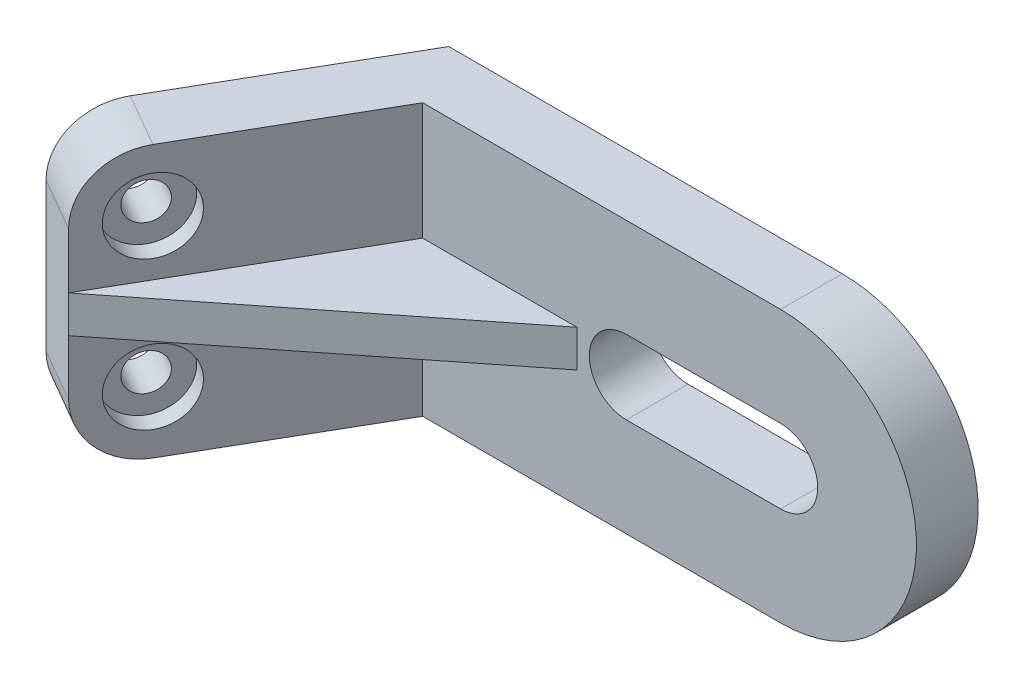
ISO-10303-21;
HEADER;
FILE_DESCRIPTION(('STEP AP214'),'2;1');
FILE_NAME('part.step','',(''),(''),'','','');
FILE_SCHEMA(('AUTOMOTIVE_DESIGN { 1 0 10303 214 1 1 1 1 }'));
ENDSEC;
DATA;
#1=APPLICATION_CONTEXT('core data for automotive mechanical design processes');
#2=APPLICATION_PROTOCOL_DEFINITION('international standard','automotive_design',2000,#1);
#3=PRODUCT_CONTEXT('',#1,'mechanical');
#4=PRODUCT('Part','Part','',(#3));
#5=PRODUCT_RELATED_PRODUCT_CATEGORY('part','',(#4));
#6=PRODUCT_DEFINITION_FORMATION('','',#4);
#7=PRODUCT_DEFINITION_CONTEXT('part definition',#1,'design');
#8=PRODUCT_DEFINITION('design','',#6,#7);
#9=PRODUCT_DEFINITION_SHAPE('','',#8);
#10=(LENGTH_UNIT() NAMED_UNIT(*) SI_UNIT(.MILLI.,.METRE.));
#11=(NAMED_UNIT(*) PLANE_ANGLE_UNIT() SI_UNIT($,.RADIAN.));
#12=(NAMED_UNIT(*) SI_UNIT($,.STERADIAN.) SOLID_ANGLE_UNIT());
#13=UNCERTAINTY_MEASURE_WITH_UNIT(LENGTH_MEASURE(1.E-05),#10,'distance_accuracy_value','');
#14=(GEOMETRIC_REPRESENTATION_CONTEXT(3) GLOBAL_UNCERTAINTY_ASSIGNED_CONTEXT((#13)) GLOBAL_UNIT_ASSIGNED_CONTEXT((#10,
#11,#12)) REPRESENTATION_CONTEXT('',''));
#15=CARTESIAN_POINT('',(0.,0.,0.));
#16=DIRECTION('',(0.,0.,1.));
#17=DIRECTION('',(1.,0.,0.));
#18=AXIS2_PLACEMENT_3D('',#15,#16,#17);
#19=CARTESIAN_POINT('',(25.,44.,10.));
#20=DIRECTION('',(0.620245802938485,0.,0.784407511397739));
#21=DIRECTION('',(0.784407511397739,0.,-0.620245802938485));
#22=AXIS2_PLACEMENT_3D('',#19,#20,#21);
#23=PLANE('',#22);
#24=DIRECTION('',(0.,-1.,0.));
#25=VECTOR('',#24,1.);
#26=CARTESIAN_POINT('',(25.,44.,10.));
#27=LINE('',#26,#25);
#28=CARTESIAN_POINT('',(25.,25.,10.));
#29=VERTEX_POINT('',#28);
#30=CARTESIAN_POINT('',(25.,19.,10.));
#31=VERTEX_POINT('',#30);
#32=EDGE_CURVE('E61',#29,#31,#27,.T.);
#33=ORIENTED_EDGE('',*,*,#32,.F.);
#34=DIRECTION('',(0.784407511397739,0.,-0.620245802938485));
#35=VECTOR('',#34,1.);
#36=CARTESIAN_POINT('',(-21.0000000000002,25.,46.3730669589463));
#37=LINE('',#36,#35);
#38=CARTESIAN_POINT('',(-21.0000000000002,25.,46.3730669589463));
#39=VERTEX_POINT('',#38);
#40=EDGE_CURVE('E161',#39,#29,#37,.T.);
#41=ORIENTED_EDGE('',*,*,#40,.F.);
#42=DIRECTION('',(0.,-1.,0.));
#43=VECTOR('',#42,1.);
#44=CARTESIAN_POINT('',(-21.0000000000002,44.,46.3730669589463));
#45=LINE('',#44,#43);
#46=CARTESIAN_POINT('',(-21.0000000000002,19.,46.3730669589463));
#47=VERTEX_POINT('',#46);
#48=EDGE_CURVE('E234',#39,#47,#45,.T.);
#49=ORIENTED_EDGE('',*,*,#48,.T.);
#50=DIRECTION('',(-0.784407511397739,0.,0.620245802938485));
#51=VECTOR('',#50,1.);
#52=CARTESIAN_POINT('',(25.,19.,10.));
#53=LINE('',#52,#51);
#54=EDGE_CURVE('E173',#31,#47,#53,.T.);
#55=ORIENTED_EDGE('',*,*,#54,.F.);
#56=EDGE_LOOP('',(#33,#41,#49,#55));
#57=FACE_BOUND('',#56,.T.);
#58=ADVANCED_FACE('F50',(#57),#23,.T.);
#59=CARTESIAN_POINT('',(0.,44.,10.));
#60=DIRECTION('',(0.,-1.,0.));
#61=DIRECTION('',(0.,0.,-1.));
#62=AXIS2_PLACEMENT_3D('',#59,#60,#61);
#63=PLANE('',#62);
#64=DIRECTION('',(0.866025403784436,0.,0.500000000000004));
#65=VECTOR('',#64,1.);
#66=CARTESIAN_POINT('',(-24.6602540378445,44.,32.7128129211019));
#67=LINE('',#66,#65);
#68=CARTESIAN_POINT('',(-24.6602540378445,44.,32.7128129211019));
#69=VERTEX_POINT('',#68);
#70=CARTESIAN_POINT('',(-16.0000000000001,44.,37.712812921102));
#71=VERTEX_POINT('',#70);
#72=EDGE_CURVE('E206',#69,#71,#67,.T.);
#73=ORIENTED_EDGE('',*,*,#72,.T.);
#74=DIRECTION('',(-0.500000000000004,0.,0.866025403784436));
#75=VECTOR('',#74,1.);
#76=CARTESIAN_POINT('',(0.,44.,10.));
#77=LINE('',#76,#75);
#78=CARTESIAN_POINT('',(0.,44.,10.));
#79=VERTEX_POINT('',#78);
#80=EDGE_CURVE('E169',#79,#71,#77,.T.);
#81=ORIENTED_EDGE('',*,*,#80,.F.);
#82=DIRECTION('',(-1.,0.,0.));
#83=VECTOR('',#82,1.);
#84=CARTESIAN_POINT('',(0.,44.,10.));
#85=LINE('',#84,#83);
#86=CARTESIAN_POINT('',(58.,44.,10.));
#87=VERTEX_POINT('',#86);
#88=EDGE_CURVE('E273',#87,#79,#85,.T.);
#89=ORIENTED_EDGE('',*,*,#88,.F.);
#90=DIRECTION('',(0.,0.,-1.));
#91=VECTOR('',#90,1.);
#92=CARTESIAN_POINT('',(58.,44.,10.));
#93=LINE('',#92,#91);
#94=CARTESIAN_POINT('',(58.,44.,0.));
#95=VERTEX_POINT('',#94);
#96=EDGE_CURVE('E57',#87,#95,#93,.T.);
#97=ORIENTED_EDGE('',*,*,#96,.T.);
#98=DIRECTION('',(-1.,0.,0.));
#99=VECTOR('',#98,1.);
#100=CARTESIAN_POINT('',(0.,44.,0.));
#101=LINE('',#100,#99);
#102=CARTESIAN_POINT('',(-5.7735026918962,44.,0.));
#103=VERTEX_POINT('',#102);
#104=EDGE_CURVE('E277',#95,#103,#101,.T.);
#105=ORIENTED_EDGE('',*,*,#104,.T.);
#106=DIRECTION('',(0.500000000000005,0.,-0.866025403784436));
#107=VECTOR('',#106,1.);
#108=CARTESIAN_POINT('',(-4.33012701892212,44.,-2.49999999999999));
#109=LINE('',#108,#107);
#110=EDGE_CURVE('E224',#69,#103,#109,.T.);
#111=ORIENTED_EDGE('',*,*,#110,.F.);
#112=EDGE_LOOP('',(#73,#81,#89,#97,#105,#111));
#113=FACE_BOUND('',#112,.T.);
#114=ADVANCED_FACE('F298',(#113),#63,.F.);
#115=CARTESIAN_POINT('',(-4.33012701892212,44.,-2.49999999999999));
#116=DIRECTION('',(-0.866025403784436,0.,-0.500000000000005));
#117=DIRECTION('',(-0.500000000000005,0.,0.866025403784436));
#118=AXIS2_PLACEMENT_3D('',#115,#116,#117);
#119=PLANE('',#118);
#120=CARTESIAN_POINT('',(-24.6602540378445,34.,32.7128129211019));
#121=DIRECTION('',(-0.866025403784436,0.,-0.500000000000005));
#122=DIRECTION('',(-0.500000000000005,0.,0.866025403784436));
#123=AXIS2_PLACEMENT_3D('',#120,#121,#122);
#124=CIRCLE('',#123,3.);
#125=CARTESIAN_POINT('',(-26.1602540378445,34.,35.3108891324552));
#126=VERTEX_POINT('',#125);
#127=EDGE_CURVE('E51',#126,#126,#124,.T.);
#128=ORIENTED_EDGE('',*,*,#127,.F.);
#129=EDGE_LOOP('',(#128));
#130=FACE_BOUND('',#129,.T.);
#131=CARTESIAN_POINT('',(-24.6602540378445,10.,32.7128129211019));
#132=DIRECTION('',(-0.866025403784436,0.,-0.500000000000005));
#133=DIRECTION('',(-0.500000000000005,0.,0.866025403784436));
#134=AXIS2_PLACEMENT_3D('',#131,#132,#133);
#135=CIRCLE('',#134,3.);
#136=CARTESIAN_POINT('',(-26.1602540378445,10.,35.3108891324552));
#137=VERTEX_POINT('',#136);
#138=EDGE_CURVE('E195',#137,#137,#135,.T.);
#139=ORIENTED_EDGE('',*,*,#138,.F.);
#140=EDGE_LOOP('',(#139));
#141=FACE_BOUND('',#140,.T.);
#142=CARTESIAN_POINT('',(-24.6602540378445,10.,32.7128129211019));
#143=DIRECTION('',(-0.866025403784436,0.,-0.500000000000004));
#144=DIRECTION('',(0.500000000000004,0.,-0.866025403784436));
#145=AXIS2_PLACEMENT_3D('',#142,#143,#144);
#146=CIRCLE('',#145,10.);
#147=CARTESIAN_POINT('',(-24.6602540378445,0.,32.7128129211019));
#148=VERTEX_POINT('',#147);
#149=CARTESIAN_POINT('',(-29.6602540378445,10.,41.3730669589463));
#150=VERTEX_POINT('',#149);
#151=EDGE_CURVE('E203',#148,#150,#146,.T.);
#152=ORIENTED_EDGE('',*,*,#151,.T.);
#153=DIRECTION('',(0.,-1.,0.));
#154=VECTOR('',#153,1.);
#155=CARTESIAN_POINT('',(-29.6602540378445,44.,41.3730669589463));
#156=LINE('',#155,#154);
#157=CARTESIAN_POINT('',(-29.6602540378445,34.,41.3730669589463));
#158=VERTEX_POINT('',#157);
#159=EDGE_CURVE('E230',#158,#150,#156,.T.);
#160=ORIENTED_EDGE('',*,*,#159,.F.);
#161=CARTESIAN_POINT('',(-24.6602540378445,34.,32.7128129211019));
#162=DIRECTION('',(-0.866025403784436,0.,-0.500000000000004));
#163=DIRECTION('',(0.500000000000004,0.,-0.866025403784436));
#164=AXIS2_PLACEMENT_3D('',#161,#162,#163);
#165=CIRCLE('',#164,10.);
#166=EDGE_CURVE('E213',#158,#69,#165,.T.);
#167=ORIENTED_EDGE('',*,*,#166,.T.);
#168=ORIENTED_EDGE('',*,*,#110,.T.);
#169=DIRECTION('',(0.,-1.,0.));
#170=VECTOR('',#169,1.);
#171=CARTESIAN_POINT('',(-5.7735026918962,44.,0.));
#172=LINE('',#171,#170);
#173=CARTESIAN_POINT('',(-5.7735026918962,0.,0.));
#174=VERTEX_POINT('',#173);
#175=EDGE_CURVE('E227',#103,#174,#172,.T.);
#176=ORIENTED_EDGE('',*,*,#175,.T.);
#177=DIRECTION('',(0.500000000000005,0.,-0.866025403784436));
#178=VECTOR('',#177,1.);
#179=CARTESIAN_POINT('',(-4.33012701892212,0.,-2.49999999999999));
#180=LINE('',#179,#178);
#181=EDGE_CURVE('E215',#148,#174,#180,.T.);
#182=ORIENTED_EDGE('',*,*,#181,.F.);
#183=EDGE_LOOP('',(#152,#160,#167,#168,#176,#182));
#184=FACE_BOUND('',#183,.T.);
#185=ADVANCED_FACE('F292',(#130,#141,#184),#119,.T.);
#186=CARTESIAN_POINT('',(-25.3301270189224,44.,43.8730669589463));
#187=DIRECTION('',(-0.500000000000004,0.,0.866025403784436));
#188=DIRECTION('',(0.866025403784436,0.,0.500000000000004));
#189=AXIS2_PLACEMENT_3D('',#186,#187,#188);
#190=PLANE('',#189);
#191=DIRECTION('',(0.866025403784436,0.,0.500000000000004));
#192=VECTOR('',#191,1.);
#193=CARTESIAN_POINT('',(-29.6602540378445,10.,41.3730669589463));
#194=LINE('',#193,#192);
#195=CARTESIAN_POINT('',(-21.0000000000002,10.,46.3730669589463));
#196=VERTEX_POINT('',#195);
#197=EDGE_CURVE('E209',#150,#196,#194,.T.);
#198=ORIENTED_EDGE('',*,*,#197,.T.);
#199=DIRECTION('',(0.,-1.,0.));
#200=VECTOR('',#199,1.);
#201=CARTESIAN_POINT('',(-21.0000000000002,19.,46.3730669589463));
#202=LINE('',#201,#200);
#203=EDGE_CURVE('E181',#47,#196,#202,.T.);
#204=ORIENTED_EDGE('',*,*,#203,.F.);
#205=ORIENTED_EDGE('',*,*,#48,.F.);
#206=CARTESIAN_POINT('',(-21.0000000000002,34.,46.3730669589463));
#207=VERTEX_POINT('',#206);
#208=EDGE_CURVE('E235',#207,#39,#45,.T.);
#209=ORIENTED_EDGE('',*,*,#208,.F.);
#210=DIRECTION('',(0.866025403784436,0.,0.500000000000004));
#211=VECTOR('',#210,1.);
#212=CARTESIAN_POINT('',(-29.6602540378445,34.,41.3730669589463));
#213=LINE('',#212,#211);
#214=EDGE_CURVE('E220',#158,#207,#213,.T.);
#215=ORIENTED_EDGE('',*,*,#214,.F.);
#216=ORIENTED_EDGE('',*,*,#159,.T.);
#217=EDGE_LOOP('',(#198,#204,#205,#209,#215,#216));
#218=FACE_BOUND('',#217,.T.);
#219=ADVANCED_FACE('F294',(#218),#190,.T.);
#220=CARTESIAN_POINT('',(0.,0.,10.));
#221=DIRECTION('',(0.,1.,0.));
#222=DIRECTION('',(0.,0.,1.));
#223=AXIS2_PLACEMENT_3D('',#220,#221,#222);
#224=PLANE('',#223);
#225=DIRECTION('',(1.,0.,0.));
#226=VECTOR('',#225,1.);
#227=CARTESIAN_POINT('',(0.,0.,10.));
#228=LINE('',#227,#226);
#229=CARTESIAN_POINT('',(0.,0.,10.));
#230=VERTEX_POINT('',#229);
#231=CARTESIAN_POINT('',(58.,0.,10.));
#232=VERTEX_POINT('',#231);
#233=EDGE_CURVE('E271',#230,#232,#228,.T.);
#234=ORIENTED_EDGE('',*,*,#233,.F.);
#235=DIRECTION('',(0.500000000000004,0.,-0.866025403784436));
#236=VECTOR('',#235,1.);
#237=CARTESIAN_POINT('',(-21.0000000000002,0.,46.3730669589463));
#238=LINE('',#237,#236);
#239=CARTESIAN_POINT('',(-16.0000000000001,0.,37.712812921102));
#240=VERTEX_POINT('',#239);
#241=EDGE_CURVE('E186',#240,#230,#238,.T.);
#242=ORIENTED_EDGE('',*,*,#241,.F.);
#243=DIRECTION('',(0.866025403784436,0.,0.500000000000004));
#244=VECTOR('',#243,1.);
#245=CARTESIAN_POINT('',(-24.6602540378445,0.,32.7128129211019));
#246=LINE('',#245,#244);
#247=EDGE_CURVE('E202',#148,#240,#246,.T.);
#248=ORIENTED_EDGE('',*,*,#247,.F.);
#249=ORIENTED_EDGE('',*,*,#181,.T.);
#250=DIRECTION('',(1.,0.,0.));
#251=VECTOR('',#250,1.);
#252=CARTESIAN_POINT('',(0.,0.,0.));
#253=LINE('',#252,#251);
#254=CARTESIAN_POINT('',(58.,0.,0.));
#255=VERTEX_POINT('',#254);
#256=EDGE_CURVE('E269',#174,#255,#253,.T.);
#257=ORIENTED_EDGE('',*,*,#256,.T.);
#258=DIRECTION('',(0.,0.,-1.));
#259=VECTOR('',#258,1.);
#260=CARTESIAN_POINT('',(58.,0.,10.));
#261=LINE('',#260,#259);
#262=EDGE_CURVE('E11',#232,#255,#261,.T.);
#263=ORIENTED_EDGE('',*,*,#262,.F.);
#264=EDGE_LOOP('',(#234,#242,#248,#249,#257,#263));
#265=FACE_BOUND('',#264,.T.);
#266=ADVANCED_FACE('F47',(#265),#224,.F.);
#267=CARTESIAN_POINT('',(0.,0.,10.));
#268=DIRECTION('',(0.,0.,-1.));
#269=DIRECTION('',(-1.,0.,0.));
#270=AXIS2_PLACEMENT_3D('',#267,#268,#269);
#271=PLANE('',#270);
#272=DIRECTION('',(1.,0.,0.));
#273=VECTOR('',#272,1.);
#274=CARTESIAN_POINT('',(33.,16.,10.));
#275=LINE('',#274,#273);
#276=CARTESIAN_POINT('',(33.,16.,10.));
#277=VERTEX_POINT('',#276);
#278=CARTESIAN_POINT('',(58.,16.,10.));
#279=VERTEX_POINT('',#278);
#280=EDGE_CURVE('E255',#277,#279,#275,.T.);
#281=ORIENTED_EDGE('',*,*,#280,.F.);
#282=CARTESIAN_POINT('',(33.,22.,10.));
#283=DIRECTION('',(0.,0.,1.));
#284=DIRECTION('',(1.,0.,0.));
#285=AXIS2_PLACEMENT_3D('',#282,#283,#284);
#286=CIRCLE('',#285,6.);
#287=CARTESIAN_POINT('',(33.,28.,10.));
#288=VERTEX_POINT('',#287);
#289=EDGE_CURVE('E75',#288,#277,#286,.T.);
#290=ORIENTED_EDGE('',*,*,#289,.F.);
#291=DIRECTION('',(-1.,0.,0.));
#292=VECTOR('',#291,1.);
#293=CARTESIAN_POINT('',(33.,28.,10.));
#294=LINE('',#293,#292);
#295=CARTESIAN_POINT('',(58.,28.,10.));
#296=VERTEX_POINT('',#295);
#297=EDGE_CURVE('E241',#296,#288,#294,.T.);
#298=ORIENTED_EDGE('',*,*,#297,.F.);
#299=CARTESIAN_POINT('',(58.,22.,10.));
#300=DIRECTION('',(0.,0.,1.));
#301=DIRECTION('',(1.,0.,0.));
#302=AXIS2_PLACEMENT_3D('',#299,#300,#301);
#303=CIRCLE('',#302,6.);
#304=EDGE_CURVE('E253',#279,#296,#303,.T.);
#305=ORIENTED_EDGE('',*,*,#304,.F.);
#306=EDGE_LOOP('',(#281,#290,#298,#305));
#307=FACE_BOUND('',#306,.T.);
#308=ORIENTED_EDGE('',*,*,#88,.T.);
#309=DIRECTION('',(0.,1.,0.));
#310=VECTOR('',#309,1.);
#311=CARTESIAN_POINT('',(0.,25.,10.));
#312=LINE('',#311,#310);
#313=CARTESIAN_POINT('',(0.,25.,10.));
#314=VERTEX_POINT('',#313);
#315=EDGE_CURVE('E156',#314,#79,#312,.T.);
#316=ORIENTED_EDGE('',*,*,#315,.F.);
#317=DIRECTION('',(-1.,0.,0.));
#318=VECTOR('',#317,1.);
#319=CARTESIAN_POINT('',(25.,25.,10.));
#320=LINE('',#319,#318);
#321=EDGE_CURVE('E153',#29,#314,#320,.T.);
#322=ORIENTED_EDGE('',*,*,#321,.F.);
#323=ORIENTED_EDGE('',*,*,#32,.T.);
#324=DIRECTION('',(1.,0.,0.));
#325=VECTOR('',#324,1.);
#326=CARTESIAN_POINT('',(0.,19.,10.));
#327=LINE('',#326,#325);
#328=CARTESIAN_POINT('',(0.,19.,10.));
#329=VERTEX_POINT('',#328);
#330=EDGE_CURVE('E332',#329,#31,#327,.T.);
#331=ORIENTED_EDGE('',*,*,#330,.F.);
#332=DIRECTION('',(0.,-1.,0.));
#333=VECTOR('',#332,1.);
#334=CARTESIAN_POINT('',(0.,19.,10.));
#335=LINE('',#334,#333);
#336=EDGE_CURVE('E184',#329,#230,#335,.T.);
#337=ORIENTED_EDGE('',*,*,#336,.T.);
#338=ORIENTED_EDGE('',*,*,#233,.T.);
#339=CARTESIAN_POINT('',(58.,22.,10.));
#340=DIRECTION('',(0.,0.,1.));
#341=DIRECTION('',(1.,0.,0.));
#342=AXIS2_PLACEMENT_3D('',#339,#340,#341);
#343=CIRCLE('',#342,22.);
#344=EDGE_CURVE('E261',#232,#87,#343,.T.);
#345=ORIENTED_EDGE('',*,*,#344,.T.);
#346=EDGE_LOOP('',(#308,#316,#322,#323,#331,#337,#338,#345));
#347=FACE_BOUND('',#346,.T.);
#348=ADVANCED_FACE('F158',(#307,#347),#271,.F.);
#349=CARTESIAN_POINT('',(0.,0.,0.));
#350=DIRECTION('',(0.,0.,-1.));
#351=DIRECTION('',(-1.,0.,0.));
#352=AXIS2_PLACEMENT_3D('',#349,#350,#351);
#353=PLANE('',#352);
#354=CARTESIAN_POINT('',(33.,22.,0.));
#355=DIRECTION('',(0.,0.,1.));
#356=DIRECTION('',(1.,0.,0.));
#357=AXIS2_PLACEMENT_3D('',#354,#355,#356);
#358=CIRCLE('',#357,6.);
#359=CARTESIAN_POINT('',(33.,28.,0.));
#360=VERTEX_POINT('',#359);
#361=CARTESIAN_POINT('',(33.,16.,0.));
#362=VERTEX_POINT('',#361);
#363=EDGE_CURVE('E240',#360,#362,#358,.T.);
#364=ORIENTED_EDGE('',*,*,#363,.T.);
#365=DIRECTION('',(1.,0.,0.));
#366=VECTOR('',#365,1.);
#367=CARTESIAN_POINT('',(33.,16.,0.));
#368=LINE('',#367,#366);
#369=CARTESIAN_POINT('',(58.,16.,0.));
#370=VERTEX_POINT('',#369);
#371=EDGE_CURVE('E239',#362,#370,#368,.T.);
#372=ORIENTED_EDGE('',*,*,#371,.T.);
#373=CARTESIAN_POINT('',(58.,22.,0.));
#374=DIRECTION('',(0.,0.,1.));
#375=DIRECTION('',(1.,0.,0.));
#376=AXIS2_PLACEMENT_3D('',#373,#374,#375);
#377=CIRCLE('',#376,6.);
#378=CARTESIAN_POINT('',(58.,28.,0.));
#379=VERTEX_POINT('',#378);
#380=EDGE_CURVE('E242',#370,#379,#377,.T.);
#381=ORIENTED_EDGE('',*,*,#380,.T.);
#382=DIRECTION('',(-1.,0.,0.));
#383=VECTOR('',#382,1.);
#384=CARTESIAN_POINT('',(33.,28.,0.));
#385=LINE('',#384,#383);
#386=EDGE_CURVE('E250',#379,#360,#385,.T.);
#387=ORIENTED_EDGE('',*,*,#386,.T.);
#388=EDGE_LOOP('',(#364,#372,#381,#387));
#389=FACE_BOUND('',#388,.T.);
#390=ORIENTED_EDGE('',*,*,#104,.F.);
#391=CARTESIAN_POINT('',(58.,22.,0.));
#392=DIRECTION('',(0.,0.,1.));
#393=DIRECTION('',(1.,0.,0.));
#394=AXIS2_PLACEMENT_3D('',#391,#392,#393);
#395=CIRCLE('',#394,22.);
#396=EDGE_CURVE('E266',#255,#95,#395,.T.);
#397=ORIENTED_EDGE('',*,*,#396,.F.);
#398=ORIENTED_EDGE('',*,*,#256,.F.);
#399=ORIENTED_EDGE('',*,*,#175,.F.);
#400=EDGE_LOOP('',(#390,#397,#398,#399));
#401=FACE_BOUND('',#400,.T.);
#402=ADVANCED_FACE('F319',(#389,#401),#353,.T.);
#403=CARTESIAN_POINT('',(58.,22.,0.));
#404=DIRECTION('',(0.,0.,1.));
#405=DIRECTION('',(1.,0.,0.));
#406=AXIS2_PLACEMENT_3D('',#403,#404,#405);
#407=CYLINDRICAL_SURFACE('',#406,22.);
#408=ORIENTED_EDGE('',*,*,#262,.T.);
#409=ORIENTED_EDGE('',*,*,#396,.T.);
#410=ORIENTED_EDGE('',*,*,#96,.F.);
#411=ORIENTED_EDGE('',*,*,#344,.F.);
#412=EDGE_LOOP('',(#408,#409,#410,#411));
#413=FACE_BOUND('',#412,.T.);
#414=ADVANCED_FACE('F341',(#413),#407,.T.);
#415=CARTESIAN_POINT('',(33.,22.,0.));
#416=DIRECTION('',(0.,0.,1.));
#417=DIRECTION('',(1.,0.,0.));
#418=AXIS2_PLACEMENT_3D('',#415,#416,#417);
#419=CYLINDRICAL_SURFACE('',#418,6.);
#420=ORIENTED_EDGE('',*,*,#289,.T.);
#421=DIRECTION('',(0.,0.,1.));
#422=VECTOR('',#421,1.);
#423=CARTESIAN_POINT('',(33.,16.,0.));
#424=LINE('',#423,#422);
#425=EDGE_CURVE('E249',#362,#277,#424,.T.);
#426=ORIENTED_EDGE('',*,*,#425,.F.);
#427=ORIENTED_EDGE('',*,*,#363,.F.);
#428=DIRECTION('',(0.,0.,1.));
#429=VECTOR('',#428,1.);
#430=CARTESIAN_POINT('',(33.,28.,0.));
#431=LINE('',#430,#429);
#432=EDGE_CURVE('E258',#360,#288,#431,.T.);
#433=ORIENTED_EDGE('',*,*,#432,.T.);
#434=EDGE_LOOP('',(#420,#426,#427,#433));
#435=FACE_BOUND('',#434,.T.);
#436=ADVANCED_FACE('F349',(#435),#419,.F.);
#437=CARTESIAN_POINT('',(33.,28.,0.));
#438=DIRECTION('',(0.,1.,0.));
#439=DIRECTION('',(0.,0.,1.));
#440=AXIS2_PLACEMENT_3D('',#437,#438,#439);
#441=PLANE('',#440);
#442=ORIENTED_EDGE('',*,*,#297,.T.);
#443=ORIENTED_EDGE('',*,*,#432,.F.);
#444=ORIENTED_EDGE('',*,*,#386,.F.);
#445=DIRECTION('',(0.,0.,1.));
#446=VECTOR('',#445,1.);
#447=CARTESIAN_POINT('',(58.,28.,0.));
#448=LINE('',#447,#446);
#449=EDGE_CURVE('E265',#379,#296,#448,.T.);
#450=ORIENTED_EDGE('',*,*,#449,.T.);
#451=EDGE_LOOP('',(#442,#443,#444,#450));
#452=FACE_BOUND('',#451,.T.);
#453=ADVANCED_FACE('F355',(#452),#441,.F.);
#454=CARTESIAN_POINT('',(58.,22.,0.));
#455=DIRECTION('',(0.,0.,1.));
#456=DIRECTION('',(1.,0.,0.));
#457=AXIS2_PLACEMENT_3D('',#454,#455,#456);
#458=CYLINDRICAL_SURFACE('',#457,6.);
#459=ORIENTED_EDGE('',*,*,#304,.T.);
#460=ORIENTED_EDGE('',*,*,#449,.F.);
#461=ORIENTED_EDGE('',*,*,#380,.F.);
#462=DIRECTION('',(0.,0.,1.));
#463=VECTOR('',#462,1.);
#464=CARTESIAN_POINT('',(58.,16.,0.));
#465=LINE('',#464,#463);
#466=EDGE_CURVE('E262',#370,#279,#465,.T.);
#467=ORIENTED_EDGE('',*,*,#466,.T.);
#468=EDGE_LOOP('',(#459,#460,#461,#467));
#469=FACE_BOUND('',#468,.T.);
#470=ADVANCED_FACE('F398',(#469),#458,.F.);
#471=CARTESIAN_POINT('',(33.,16.,0.));
#472=DIRECTION('',(0.,-1.,0.));
#473=DIRECTION('',(0.,0.,-1.));
#474=AXIS2_PLACEMENT_3D('',#471,#472,#473);
#475=PLANE('',#474);
#476=ORIENTED_EDGE('',*,*,#280,.T.);
#477=ORIENTED_EDGE('',*,*,#466,.F.);
#478=ORIENTED_EDGE('',*,*,#371,.F.);
#479=ORIENTED_EDGE('',*,*,#425,.T.);
#480=EDGE_LOOP('',(#476,#477,#478,#479));
#481=FACE_BOUND('',#480,.T.);
#482=ADVANCED_FACE('F394',(#481),#475,.F.);
#483=CARTESIAN_POINT('',(-24.6602540378445,34.,32.7128129211019));
#484=DIRECTION('',(0.866025403784436,0.,0.500000000000004));
#485=DIRECTION('',(0.500000000000004,0.,-0.866025403784436));
#486=AXIS2_PLACEMENT_3D('',#483,#484,#485);
#487=CYLINDRICAL_SURFACE('',#486,10.);
#488=CARTESIAN_POINT('',(-16.0000000000001,34.,37.712812921102));
#489=DIRECTION('',(-0.866025403784436,0.,-0.500000000000004));
#490=DIRECTION('',(0.500000000000004,0.,-0.866025403784436));
#491=AXIS2_PLACEMENT_3D('',#488,#489,#490);
#492=CIRCLE('',#491,10.);
#493=EDGE_CURVE('E196',#207,#71,#492,.T.);
#494=ORIENTED_EDGE('',*,*,#493,.T.);
#495=ORIENTED_EDGE('',*,*,#72,.F.);
#496=ORIENTED_EDGE('',*,*,#166,.F.);
#497=ORIENTED_EDGE('',*,*,#214,.T.);
#498=EDGE_LOOP('',(#494,#495,#496,#497));
#499=FACE_BOUND('',#498,.T.);
#500=ADVANCED_FACE('F308',(#499),#487,.T.);
#501=CARTESIAN_POINT('',(-24.6602540378445,10.,32.7128129211019));
#502=DIRECTION('',(0.866025403784436,0.,0.500000000000004));
#503=DIRECTION('',(0.500000000000004,0.,-0.866025403784436));
#504=AXIS2_PLACEMENT_3D('',#501,#502,#503);
#505=CYLINDRICAL_SURFACE('',#504,10.);
#506=CARTESIAN_POINT('',(-16.0000000000001,10.,37.712812921102));
#507=DIRECTION('',(-0.866025403784436,0.,-0.500000000000004));
#508=DIRECTION('',(0.500000000000004,0.,-0.866025403784436));
#509=AXIS2_PLACEMENT_3D('',#506,#507,#508);
#510=CIRCLE('',#509,10.);
#511=EDGE_CURVE('E204',#240,#196,#510,.T.);
#512=ORIENTED_EDGE('',*,*,#511,.T.);
#513=ORIENTED_EDGE('',*,*,#197,.F.);
#514=ORIENTED_EDGE('',*,*,#151,.F.);
#515=ORIENTED_EDGE('',*,*,#247,.T.);
#516=EDGE_LOOP('',(#512,#513,#514,#515));
#517=FACE_BOUND('',#516,.T.);
#518=ADVANCED_FACE('F324',(#517),#505,.T.);
#519=CARTESIAN_POINT('',(-18.5980762113534,10.,36.2128129211019));
#520=DIRECTION('',(0.866025403784436,0.,0.500000000000004));
#521=DIRECTION('',(0.500000000000004,0.,-0.866025403784436));
#522=AXIS2_PLACEMENT_3D('',#519,#520,#521);
#523=CYLINDRICAL_SURFACE('',#522,6.);
#524=CARTESIAN_POINT('',(-18.5980762113534,10.,36.2128129211019));
#525=DIRECTION('',(0.866025403784436,0.,0.500000000000004));
#526=DIRECTION('',(0.500000000000004,0.,-0.866025403784436));
#527=AXIS2_PLACEMENT_3D('',#524,#525,#526);
#528=CIRCLE('',#527,6.);
#529=CARTESIAN_POINT('',(-15.5980762113534,10.,31.0166604983953));
#530=VERTEX_POINT('',#529);
#531=EDGE_CURVE('E200',#530,#530,#528,.T.);
#532=ORIENTED_EDGE('',*,*,#531,.F.);
#533=EDGE_LOOP('',(#532));
#534=FACE_BOUND('',#533,.T.);
#535=CARTESIAN_POINT('',(-16.0000000000001,10.,37.712812921102));
#536=DIRECTION('',(-0.866025403784436,0.,-0.500000000000004));
#537=DIRECTION('',(-0.500000000000004,0.,0.866025403784436));
#538=AXIS2_PLACEMENT_3D('',#535,#536,#537);
#539=CIRCLE('',#538,6.);
#540=CARTESIAN_POINT('',(-19.0000000000002,10.,42.9089653438086));
#541=VERTEX_POINT('',#540);
#542=EDGE_CURVE('E174',#541,#541,#539,.F.);
#543=ORIENTED_EDGE('',*,*,#542,.T.);
#544=EDGE_LOOP('',(#543));
#545=FACE_BOUND('',#544,.T.);
#546=ADVANCED_FACE('F385',(#534,#545),#523,.F.);
#547=CARTESIAN_POINT('',(-18.5980762113534,10.,36.2128129211019));
#548=DIRECTION('',(0.866025403784436,0.,0.500000000000004));
#549=DIRECTION('',(0.500000000000004,0.,-0.866025403784436));
#550=AXIS2_PLACEMENT_3D('',#547,#548,#549);
#551=PLANE('',#550);
#552=CARTESIAN_POINT('',(-18.5980762113534,10.,36.2128129211019));
#553=DIRECTION('',(0.866025403784436,0.,0.500000000000004));
#554=DIRECTION('',(0.500000000000004,0.,-0.866025403784436));
#555=AXIS2_PLACEMENT_3D('',#552,#553,#554);
#556=CIRCLE('',#555,3.);
#557=CARTESIAN_POINT('',(-17.0980762113534,10.,33.6147367097486));
#558=VERTEX_POINT('',#557);
#559=EDGE_CURVE('E172',#558,#558,#556,.T.);
#560=ORIENTED_EDGE('',*,*,#559,.F.);
#561=EDGE_LOOP('',(#560));
#562=FACE_BOUND('',#561,.T.);
#563=ORIENTED_EDGE('',*,*,#531,.T.);
#564=EDGE_LOOP('',(#563));
#565=FACE_BOUND('',#564,.T.);
#566=ADVANCED_FACE('F377',(#562,#565),#551,.T.);
#567=CARTESIAN_POINT('',(-18.5980762113534,34.,36.2128129211019));
#568=DIRECTION('',(0.866025403784436,0.,0.500000000000004));
#569=DIRECTION('',(0.500000000000004,0.,-0.866025403784436));
#570=AXIS2_PLACEMENT_3D('',#567,#568,#569);
#571=CYLINDRICAL_SURFACE('',#570,5.99999999999999);
#572=CARTESIAN_POINT('',(-18.5980762113534,34.,36.2128129211019));
#573=DIRECTION('',(0.866025403784436,0.,0.500000000000004));
#574=DIRECTION('',(0.500000000000004,0.,-0.866025403784436));
#575=AXIS2_PLACEMENT_3D('',#572,#573,#574);
#576=CIRCLE('',#575,5.99999999999999);
#577=CARTESIAN_POINT('',(-15.5980762113534,34.,31.0166604983953));
#578=VERTEX_POINT('',#577);
#579=EDGE_CURVE('E191',#578,#578,#576,.T.);
#580=ORIENTED_EDGE('',*,*,#579,.F.);
#581=EDGE_LOOP('',(#580));
#582=FACE_BOUND('',#581,.T.);
#583=CARTESIAN_POINT('',(-16.0000000000001,34.,37.712812921102));
#584=DIRECTION('',(-0.866025403784436,0.,-0.500000000000004));
#585=DIRECTION('',(-0.500000000000004,0.,0.866025403784436));
#586=AXIS2_PLACEMENT_3D('',#583,#584,#585);
#587=CIRCLE('',#586,5.99999999999999);
#588=CARTESIAN_POINT('',(-19.0000000000002,34.,42.9089653438086));
#589=VERTEX_POINT('',#588);
#590=EDGE_CURVE('E190',#589,#589,#587,.F.);
#591=ORIENTED_EDGE('',*,*,#590,.T.);
#592=EDGE_LOOP('',(#591));
#593=FACE_BOUND('',#592,.T.);
#594=ADVANCED_FACE('F372',(#582,#593),#571,.F.);
#595=CARTESIAN_POINT('',(-18.5980762113534,34.,36.2128129211019));
#596=DIRECTION('',(0.866025403784436,0.,0.500000000000004));
#597=DIRECTION('',(0.500000000000004,0.,-0.866025403784436));
#598=AXIS2_PLACEMENT_3D('',#595,#596,#597);
#599=PLANE('',#598);
#600=CARTESIAN_POINT('',(-18.5980762113534,34.,36.2128129211019));
#601=DIRECTION('',(0.866025403784436,0.,0.500000000000004));
#602=DIRECTION('',(0.500000000000004,0.,-0.866025403784436));
#603=AXIS2_PLACEMENT_3D('',#600,#601,#602);
#604=CIRCLE('',#603,3.);
#605=CARTESIAN_POINT('',(-17.0980762113534,34.,33.6147367097486));
#606=VERTEX_POINT('',#605);
#607=EDGE_CURVE('E178',#606,#606,#604,.T.);
#608=ORIENTED_EDGE('',*,*,#607,.F.);
#609=EDGE_LOOP('',(#608));
#610=FACE_BOUND('',#609,.T.);
#611=ORIENTED_EDGE('',*,*,#579,.T.);
#612=EDGE_LOOP('',(#611));
#613=FACE_BOUND('',#612,.T.);
#614=ADVANCED_FACE('F371',(#610,#613),#599,.T.);
#615=CARTESIAN_POINT('',(-27.2583302491978,10.,31.2128129211019));
#616=DIRECTION('',(0.866025403784436,0.,0.500000000000004));
#617=DIRECTION('',(0.500000000000004,0.,-0.866025403784436));
#618=AXIS2_PLACEMENT_3D('',#615,#616,#617);
#619=CYLINDRICAL_SURFACE('',#618,3.);
#620=ORIENTED_EDGE('',*,*,#138,.T.);
#621=EDGE_LOOP('',(#620));
#622=FACE_BOUND('',#621,.T.);
#623=ORIENTED_EDGE('',*,*,#559,.T.);
#624=EDGE_LOOP('',(#623));
#625=FACE_BOUND('',#624,.T.);
#626=ADVANCED_FACE('F368',(#622,#625),#619,.F.);
#627=CARTESIAN_POINT('',(-27.2583302491978,34.,31.2128129211019));
#628=DIRECTION('',(0.866025403784436,0.,0.500000000000004));
#629=DIRECTION('',(0.500000000000004,0.,-0.866025403784436));
#630=AXIS2_PLACEMENT_3D('',#627,#628,#629);
#631=CYLINDRICAL_SURFACE('',#630,3.);
#632=ORIENTED_EDGE('',*,*,#127,.T.);
#633=EDGE_LOOP('',(#632));
#634=FACE_BOUND('',#633,.T.);
#635=ORIENTED_EDGE('',*,*,#607,.T.);
#636=EDGE_LOOP('',(#635));
#637=FACE_BOUND('',#636,.T.);
#638=ADVANCED_FACE('F287',(#634,#637),#631,.F.);
#639=CARTESIAN_POINT('',(-21.0000000000002,19.,46.3730669589463));
#640=DIRECTION('',(-0.866025403784436,0.,-0.500000000000005));
#641=DIRECTION('',(-0.500000000000005,0.,0.866025403784436));
#642=AXIS2_PLACEMENT_3D('',#639,#640,#641);
#643=PLANE('',#642);
#644=ORIENTED_EDGE('',*,*,#241,.T.);
#645=ORIENTED_EDGE('',*,*,#336,.F.);
#646=DIRECTION('',(0.500000000000004,0.,-0.866025403784436));
#647=VECTOR('',#646,1.);
#648=CARTESIAN_POINT('',(-21.0000000000002,19.,46.3730669589463));
#649=LINE('',#648,#647);
#650=EDGE_CURVE('E327',#47,#329,#649,.T.);
#651=ORIENTED_EDGE('',*,*,#650,.F.);
#652=ORIENTED_EDGE('',*,*,#203,.T.);
#653=ORIENTED_EDGE('',*,*,#511,.F.);
#654=EDGE_LOOP('',(#644,#645,#651,#652,#653));
#655=FACE_BOUND('',#654,.T.);
#656=ORIENTED_EDGE('',*,*,#542,.F.);
#657=EDGE_LOOP('',(#656));
#658=FACE_BOUND('',#657,.T.);
#659=ADVANCED_FACE('F323',(#655,#658),#643,.F.);
#660=CARTESIAN_POINT('',(0.,19.,0.));
#661=DIRECTION('',(0.,-1.,0.));
#662=DIRECTION('',(0.,0.,-1.));
#663=AXIS2_PLACEMENT_3D('',#660,#661,#662);
#664=PLANE('',#663);
#665=ORIENTED_EDGE('',*,*,#650,.T.);
#666=ORIENTED_EDGE('',*,*,#330,.T.);
#667=ORIENTED_EDGE('',*,*,#54,.T.);
#668=EDGE_LOOP('',(#665,#666,#667));
#669=FACE_BOUND('',#668,.T.);
#670=ADVANCED_FACE('F439',(#669),#664,.T.);
#671=CARTESIAN_POINT('',(0.,25.,10.));
#672=DIRECTION('',(-0.866025403784436,0.,-0.500000000000004));
#673=DIRECTION('',(-0.500000000000004,0.,0.866025403784436));
#674=AXIS2_PLACEMENT_3D('',#671,#672,#673);
#675=PLANE('',#674);
#676=ORIENTED_EDGE('',*,*,#208,.T.);
#677=DIRECTION('',(-0.500000000000004,0.,0.866025403784436));
#678=VECTOR('',#677,1.);
#679=CARTESIAN_POINT('',(0.,25.,10.));
#680=LINE('',#679,#678);
#681=EDGE_CURVE('E162',#314,#39,#680,.T.);
#682=ORIENTED_EDGE('',*,*,#681,.F.);
#683=ORIENTED_EDGE('',*,*,#315,.T.);
#684=ORIENTED_EDGE('',*,*,#80,.T.);
#685=ORIENTED_EDGE('',*,*,#493,.F.);
#686=EDGE_LOOP('',(#676,#682,#683,#684,#685));
#687=FACE_BOUND('',#686,.T.);
#688=ORIENTED_EDGE('',*,*,#590,.F.);
#689=EDGE_LOOP('',(#688));
#690=FACE_BOUND('',#689,.T.);
#691=ADVANCED_FACE('F338',(#687,#690),#675,.F.);
#692=CARTESIAN_POINT('',(0.,25.,0.));
#693=DIRECTION('',(0.,1.,0.));
#694=DIRECTION('',(0.,0.,1.));
#695=AXIS2_PLACEMENT_3D('',#692,#693,#694);
#696=PLANE('',#695);
#697=ORIENTED_EDGE('',*,*,#40,.T.);
#698=ORIENTED_EDGE('',*,*,#321,.T.);
#699=ORIENTED_EDGE('',*,*,#681,.T.);
#700=EDGE_LOOP('',(#697,#698,#699));
#701=FACE_BOUND('',#700,.T.);
#702=ADVANCED_FACE('F168',(#701),#696,.T.);
#703=CLOSED_SHELL('',(#58,#114,#185,#219,#266,#348,#402,#414,#436,#453,#470,#482,#500,#518,#546,
#566,#594,#614,#626,#638,#659,#670,#691,#702));
#704=MANIFOLD_SOLID_BREP('B2',#703);
#705=ADVANCED_BREP_SHAPE_REPRESENTATION('',(#18,#704),#14);
#706=SHAPE_DEFINITION_REPRESENTATION(#9,#705);
ENDSEC;
END-ISO-10303-21;
